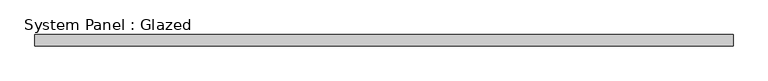
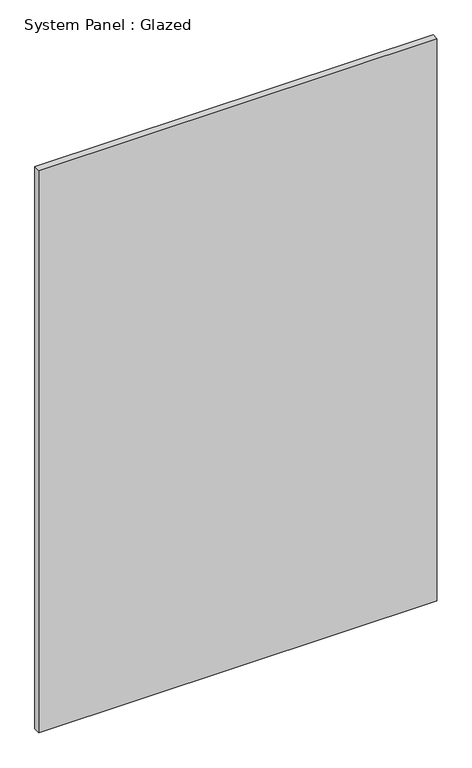
"""IFC4 building model written with IfcOpenShell, lengths in millimetres: plate geometry, System Panel : Glazed."""

from ifc_helpers import new_model, si_unit, origin, origin_with_axes, place, context, project, spatial, polyline, outline, extrude, source, transform, mapped, element, save


def system_panel_glazed_87f78641(model_context):
    return source(origin(), model_context, "Body", "SweptSolid", [
        extrude(outline(polyline([(787.4, 19.05), (-787.4, 19.05), (-787.4, 44.45), (787.4, 44.45), (787.4, 19.05)])), origin_with_axes(), (0.0, 0.0, 1.0), 2351.1880434),
    ])


if __name__ == "__main__":
    model = new_model("IFC4")
    model_context = context("Model", 3, world=origin())
    ifc_project = project(units=[si_unit("LENGTHUNIT", "METRE", prefix="MILLI")], contexts=[model_context])
    site = spatial("IfcSite", under=ifc_project)
    building = spatial("IfcBuilding", under=site)
    placement = place(None, origin())
    system_panel_glazed_shape = system_panel_glazed_87f78641(model_context)
    element("IfcPlate", 1, ObjectType="System Panel : Glazed", at=placement, inside=building, context=model_context, shape_type="MappedRepresentation", body=[
        mapped(system_panel_glazed_shape, transform((0.0, 0.0, 0.0), x_axis=(1.0, 0.0, 0.0), y_axis=(0.0, 1.0, 0.0), z_axis=(0.0, 0.0, 1.0))),
    ])
    save(model, "model.ifc")

# Revit data of these elements
# Type "System Panel : Glazed"
#   Construction Type Id = "GSP4R"
#   Analytic Construction = "1/8 in Pilkington single glazing"
#   Visual Light Transmittance = 0.9
#   Solar Heat Gain Coefficient = 0.86
#   Heat Transfer Coefficient (U) = 1.18115 BTU/(h·ft²·°F)
# Element 1 (IfcPlate, "System Panel : Glazed")
#   Materials on its faces: "Glass"
# Materials
#   "Glass": class "Glass", colour RGB 0 128 192, transparency 0.75, Description = "Soda Lime Glass", Cost = 0
